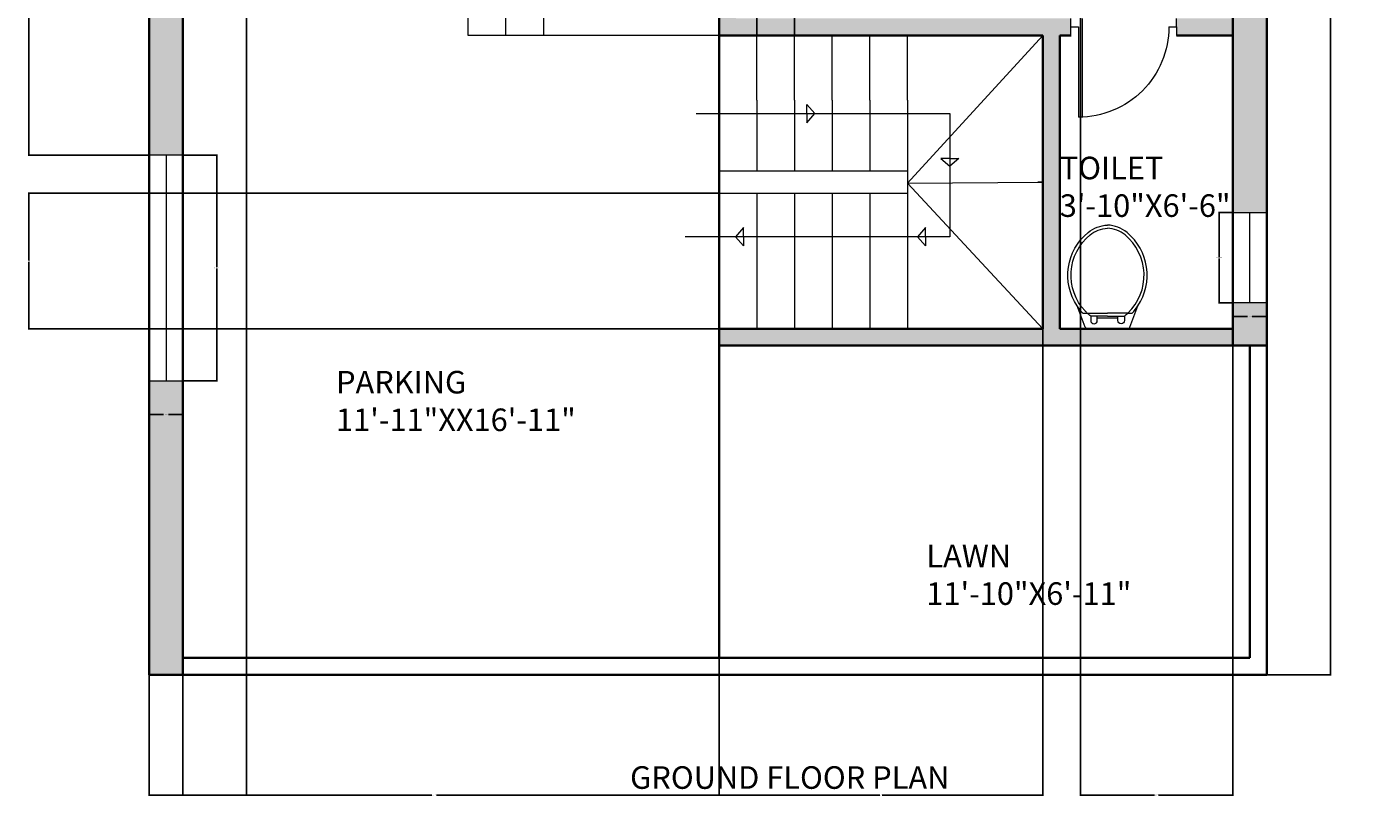
# Model space of a CAD drawing. Units: inches. Extents: x -13 to 349, y -556 to 61.
# Tile 1 of 6: x -13 to 345, y -556 to -351. Entities that reach past the tile are written whole.
import ezdxf

# ---------------------------------------------------------------- set-up
doc = ezdxf.new("R2010")
doc.units = ezdxf.units.IN
doc.header["$MEASUREMENT"] = 0
for name, color, linetype, lineweight in [('A-ANNO-DIMS', 2, 'Continuous', 18), ('A-ANNO-SYMB', 7, 'Continuous', 13), ('A-ANNO-TEXT', 7, 'Continuous', 25), ('A-AREA-IDEN', 7, 'Continuous', 18), ('A-DOOR', 3, 'Continuous', 20), ('A-FLOR-STRS', 7, 'Continuous', 20), ('A-GLAZ', 5, 'Continuous', 18), ('A-WALL', 7, 'Continuous', 35), ('A-WALL-PATT', 8, 'Continuous', 13), ('WC-Detail_dwgmodels.com', 251, 'Continuous', 13), ('WC-Outline_dwgmodels.com', 250, 'Continuous', 18)]:
    doc.layers.add(name, color=color, linetype=linetype, lineweight=lineweight)
doc.styles.get("Standard").update_dxf_attribs({"font": 'arial.ttf'})
doc.dimstyles.get("Standard").update_dxf_attribs({"dimtxt": 0.18, "dimasz": 0.18, "dimexe": 0.18, "dimexo": 0.0625, "dimgap": 0.09, "dimtad": 0, "dimtih": 1, "dimtoh": 1, "dimdec": 0, "dimzin": 0, "dimdsep": 46, "dimlunit": 3, "dimtxsty": 'Standard', "dimcen": 0.09, "dimadec": 0, "dimazin": 0, "dimtfac": 1, "dimtdec": 0, "dimtofl": 0, "dimtmove": 0, "dimatfit": 3, "dimfxl": 1, "dimtolj": 1, "dimtzin": 0, "dimarcsym": 0})

# ---------------------------------------------------------------- blocks, each defined once
blk = doc.blocks.new('*D3')
at = {"layer": 'A-ANNO-DIMS', "color": 0, "lineweight": -2, "transparency": 16777216}
for p, q in [((316.82, 8.29), (333.9, 8.29)), ((333.72, 8.11), (333.72, -254.62)), ((333.72, -523.53), (333.72, -260.8)), ((316.82, -523.71), (333.9, -523.71))]:
    blk.add_line(p, q, dxfattribs=at)
at = {"layer": 'A-ANNO-DIMS', "color": 0, "transparency": 16777216}
for points in [[(333.69, 8.11), (333.75, 8.11), (333.72, 8.29)], [(333.69, -523.53), (333.75, -523.53), (333.72, -523.71)]]:
    blk.add_solid(points, dxfattribs=at)
at = {"layer": 'Defpoints', "color": 0, "transparency": 16777216}
for p in [(316.76, 8.29), (316.76, -523.71), (333.72, -523.71)]:
    blk.add_point(p, dxfattribs=at)
at = {"layer": 'A-ANNO-DIMS', "color": 0, "transparency": 16777216, "insert": (333.72, -257.71), "char_height": 6, "attachment_point": 5}
blk.add_mtext('\\A1;44\'-4"', dxfattribs=at)
blk = doc.blocks.new('DOOR-SWING-24IN')
for p, q in [((4.5, 28), (0, 28)), ((2.25, 28), (2.25, 26)), ((2.25, 26), (26.25, 26)), ((0, 25), (26.25, 25)), ((2.25, 2), (2.25, 0)), ((2.25, 0), (0, 0)), ((2.25, 0), (4.5, 0))]:
    blk.add_line(p, q)
blk.add_arc((2.25, 26), 24, 270, 0)
blk = doc.blocks.new('WIN-60IN-D9')
for p, q in [((0, 60), (0, 0)), ((9, 60), (0, 60)), ((4.5, 60), (4.5, 0)), ((9, 0), (9, 60)), ((0, 0), (9, 0))]:
    blk.add_line(p, q)
blk = doc.blocks.new('WIN-24IN-D9')
for p, q in [((0, 9), (24, 9)), ((0, 0), (0, 9)), ((24, 9), (24, 0)), ((0, 4.5), (24, 4.5)), ((24, 0), (0, 0))]:
    blk.add_line(p, q)
blk = doc.blocks.new('STAIR-DIRECTION-HEAD')
for p, q in [((2.12, 4.81), (0, 2.4)), ((2.12, 2.4), (2.12, 4.81)), ((2.12, 0), (0, 2.4)), ((2.12, 2.4), (2.12, 0))]:
    blk.add_line(p, q)
blk = doc.blocks.new('*D18')
at = {"layer": 'A-ANNO-DIMS', "color": 0, "lineweight": -2, "transparency": 16777216}
for p, q in [((28.82, -385.56), (37.94, -385.56)), ((37.76, -385.74), (37.76, -415.38)), ((37.76, -445.38), (37.76, -415.74)), ((28.82, -445.56), (37.94, -445.56))]:
    blk.add_line(p, q, dxfattribs=at)
at = {"layer": 'A-ANNO-DIMS', "color": 0, "transparency": 16777216}
for points in [[(37.73, -385.74), (37.79, -385.74), (37.76, -385.56)], [(37.73, -445.38), (37.79, -445.38), (37.76, -445.56)]]:
    blk.add_solid(points, dxfattribs=at)
at = {"layer": 'Defpoints', "color": 0, "transparency": 16777216}
for p in [(28.76, -385.56), (37.76, -385.56), (28.76, -445.56)]:
    blk.add_point(p, dxfattribs=at)
at = {"layer": 'A-ANNO-DIMS', "color": 0, "transparency": 16777216, "insert": (37.76, -415.56), "char_height": 0.18, "attachment_point": 5}
blk.add_mtext('\\A1;W1 5\'-0" TYP.', dxfattribs=at)
blk = doc.blocks.new('*D19')
at = {"layer": 'A-ANNO-DIMS', "color": 0, "lineweight": -2, "transparency": 16777216}
for p, q in [((19.76, -445.62), (19.76, -454.74)), ((28.76, -445.62), (28.76, -454.74)), ((19.94, -454.56), (23.62, -454.56)), ((28.58, -454.56), (24.89, -454.56))]:
    blk.add_line(p, q, dxfattribs=at)
at = {"layer": 'A-ANNO-DIMS', "color": 0, "transparency": 16777216}
for points in [[(19.94, -454.53), (19.94, -454.59), (19.76, -454.56)], [(28.58, -454.53), (28.58, -454.59), (28.76, -454.56)]]:
    blk.add_solid(points, dxfattribs=at)
at = {"layer": 'Defpoints', "color": 0, "transparency": 16777216}
for p in [(19.76, -445.56), (28.76, -445.56), (28.76, -454.56)]:
    blk.add_point(p, dxfattribs=at)
at = {"layer": 'A-ANNO-DIMS', "color": 0, "transparency": 16777216, "insert": (24.26, -454.56), "char_height": 0.18, "attachment_point": 5}
blk.add_mtext('\\A1;0\'-9" TYP.', dxfattribs=at)
blk = doc.blocks.new('*D20')
at = {"layer": 'A-ANNO-DIMS', "color": 0, "lineweight": -2, "transparency": 16777216}
for p, q in [((307.69, -400.85), (303.98, -400.85)), ((304.16, -401.03), (304.16, -412.67)), ((304.16, -424.67), (304.16, -413.03)), ((307.69, -424.85), (303.98, -424.85))]:
    blk.add_line(p, q, dxfattribs=at)
at = {"layer": 'A-ANNO-DIMS', "color": 0, "transparency": 16777216}
for points in [[(304.13, -401.03), (304.19, -401.03), (304.16, -400.85)], [(304.13, -424.67), (304.19, -424.67), (304.16, -424.85)]]:
    blk.add_solid(points, dxfattribs=at)
at = {"layer": 'Defpoints', "color": 0, "transparency": 16777216}
for p in [(304.16, -400.85), (307.76, -400.85), (307.76, -424.85)]:
    blk.add_point(p, dxfattribs=at)
at = {"layer": 'A-ANNO-DIMS', "color": 0, "transparency": 16777216, "insert": (304.16, -412.85), "char_height": 0.18, "attachment_point": 5}
blk.add_mtext('\\A1;W2 2\'-0" TYP.', dxfattribs=at)
blk = doc.blocks.new('*D21')
at = {"layer": 'A-ANNO-DIMS', "color": 0, "lineweight": -2, "transparency": 16777216}
for p, q in [((307.76, -424.91), (307.76, -428.63)), ((316.76, -424.91), (316.76, -428.63)), ((307.94, -428.45), (311.62, -428.45)), ((316.58, -428.45), (312.89, -428.45))]:
    blk.add_line(p, q, dxfattribs=at)
at = {"layer": 'A-ANNO-DIMS', "color": 0, "transparency": 16777216}
for points in [[(307.94, -428.42), (307.94, -428.48), (307.76, -428.45)], [(316.58, -428.42), (316.58, -428.48), (316.76, -428.45)]]:
    blk.add_solid(points, dxfattribs=at)
at = {"layer": 'Defpoints', "color": 0, "transparency": 16777216}
for p in [(307.76, -424.85), (316.76, -424.85), (307.76, -428.45)]:
    blk.add_point(p, dxfattribs=at)
at = {"layer": 'A-ANNO-DIMS', "color": 0, "transparency": 16777216, "insert": (312.26, -428.45), "char_height": 0.18, "attachment_point": 5}
blk.add_mtext('\\A1;0\'-9" TYP.', dxfattribs=at)
blk = doc.blocks.new('*D34')
at = {"layer": 'A-ANNO-DIMS', "color": 0, "lineweight": -2, "transparency": 16777216}
for p, q in [((267.26, -200.78), (267.26, -555.89)), ((307.76, -200.78), (307.76, -555.89)), ((267.44, -555.71), (286.97, -555.71)), ((307.58, -555.71), (288.04, -555.71))]:
    blk.add_line(p, q, dxfattribs=at)
at = {"layer": 'A-ANNO-DIMS', "color": 0, "transparency": 16777216}
for points in [[(267.44, -555.68), (267.44, -555.74), (267.26, -555.71)], [(307.58, -555.68), (307.58, -555.74), (307.76, -555.71)]]:
    blk.add_solid(points, dxfattribs=at)
at = {"layer": 'Defpoints', "color": 0, "transparency": 16777216}
for p in [(267.26, -200.71), (307.76, -200.71), (307.76, -555.71)]:
    blk.add_point(p, dxfattribs=at)
at = {"layer": 'A-ANNO-DIMS', "color": 0, "transparency": 16777216, "insert": (287.51, -555.71), "char_height": 0.18, "attachment_point": 5}
blk.add_mtext('\\A1;3\'-4 1/2"', dxfattribs=at)
blk = doc.blocks.new('*D35')
at = {"layer": 'A-ANNO-DIMS', "color": 0, "lineweight": -2, "transparency": 16777216}
for p, q in [((171.26, -431.78), (171.26, -555.89)), ((257.26, -431.78), (257.26, -555.89)), ((171.44, -555.71), (213.93, -555.71)), ((257.08, -555.71), (214.58, -555.71))]:
    blk.add_line(p, q, dxfattribs=at)
at = {"layer": 'A-ANNO-DIMS', "color": 0, "transparency": 16777216}
for points in [[(171.44, -555.68), (171.44, -555.74), (171.26, -555.71)], [(257.08, -555.68), (257.08, -555.74), (257.26, -555.71)]]:
    blk.add_solid(points, dxfattribs=at)
at = {"layer": 'Defpoints', "color": 0, "transparency": 16777216}
for p in [(171.26, -431.71), (257.26, -431.71), (257.26, -555.71)]:
    blk.add_point(p, dxfattribs=at)
at = {"layer": 'A-ANNO-DIMS', "color": 0, "transparency": 16777216, "insert": (214.26, -555.71), "char_height": 0.18, "attachment_point": 5}
blk.add_mtext('\\A1;7\'-2"', dxfattribs=at)
blk = doc.blocks.new('*D36')
at = {"layer": 'A-ANNO-DIMS', "color": 0, "lineweight": -2, "transparency": 16777216}
for p, q in [((171.19, -395.71), (-12.42, -395.71)), ((-12.24, -395.89), (-12.24, -413.53)), ((-12.24, -431.53), (-12.24, -413.9)), ((171.19, -431.71), (-12.42, -431.71))]:
    blk.add_line(p, q, dxfattribs=at)
at = {"layer": 'A-ANNO-DIMS', "color": 0, "transparency": 16777216}
for points in [[(-12.27, -395.89), (-12.21, -395.89), (-12.24, -395.71)], [(-12.27, -431.53), (-12.21, -431.53), (-12.24, -431.71)]]:
    blk.add_solid(points, dxfattribs=at)
at = {"layer": 'Defpoints', "color": 0, "transparency": 16777216}
for p in [(-12.24, -395.71), (171.26, -395.71), (171.26, -431.71)]:
    blk.add_point(p, dxfattribs=at)
at = {"layer": 'A-ANNO-DIMS', "color": 0, "transparency": 16777216, "insert": (-12.24, -413.71), "char_height": 0.18, "attachment_point": 5}
blk.add_mtext('\\A1;3\'-0"', dxfattribs=at)
blk = doc.blocks.new('*D37')
at = {"layer": 'A-ANNO-DIMS', "color": 0, "lineweight": -2, "transparency": 16777216}
for p, q in [((181.26, -353.65), (181.26, 40.47)), ((181.44, 40.29), (185.86, 40.29)), ((191.08, 40.29), (186.65, 40.29)), ((191.26, -353.65), (191.26, 40.47))]:
    blk.add_line(p, q, dxfattribs=at)
at = {"layer": 'A-ANNO-DIMS', "color": 0, "transparency": 16777216}
for points in [[(181.44, 40.32), (181.44, 40.26), (181.26, 40.29)], [(191.08, 40.32), (191.08, 40.26), (191.26, 40.29)]]:
    blk.add_solid(points, dxfattribs=at)
at = {"layer": 'Defpoints', "color": 0, "transparency": 16777216}
for p in [(191.26, 40.29), (181.26, -353.71), (191.26, -353.71)]:
    blk.add_point(p, dxfattribs=at)
at = {"layer": 'A-ANNO-DIMS', "color": 0, "transparency": 16777216, "insert": (186.26, 40.29), "char_height": 0.18, "attachment_point": 5}
blk.add_mtext('\\A1;0\'-10"', dxfattribs=at)
blk = doc.blocks.new('*D38')
at = {"layer": 'A-ANNO-DIMS', "color": 0, "lineweight": -2, "transparency": 16777216}
for p, q in [((28.76, -144.78), (28.76, -555.89)), ((45.63, -144.78), (45.63, -555.89)), ((28.94, -555.71), (36.87, -555.71)), ((45.45, -555.71), (37.51, -555.71))]:
    blk.add_line(p, q, dxfattribs=at)
at = {"layer": 'A-ANNO-DIMS', "color": 0, "transparency": 16777216}
for points in [[(28.94, -555.68), (28.94, -555.74), (28.76, -555.71)], [(45.45, -555.68), (45.45, -555.74), (45.63, -555.71)]]:
    blk.add_solid(points, dxfattribs=at)
at = {"layer": 'Defpoints', "color": 0, "transparency": 16777216}
for p in [(28.76, -144.71), (45.63, -144.71), (45.63, -555.71)]:
    blk.add_point(p, dxfattribs=at)
at = {"layer": 'A-ANNO-DIMS', "color": 0, "transparency": 16777216, "insert": (37.19, -555.71), "char_height": 0.18, "attachment_point": 5}
blk.add_mtext('\\A1;1\'-5"', dxfattribs=at)
blk = doc.blocks.new('*D46')
at = {"layer": 'A-ANNO-DIMS', "color": 0, "lineweight": -2, "transparency": 16777216}
for p, q in [((19.69, -307.06), (-12.42, -307.06)), ((-12.24, -307.24), (-12.24, -346.13)), ((-12.24, -385.38), (-12.24, -346.49)), ((19.69, -385.56), (-12.42, -385.56))]:
    blk.add_line(p, q, dxfattribs=at)
at = {"layer": 'A-ANNO-DIMS', "color": 0, "transparency": 16777216}
for points in [[(-12.27, -307.24), (-12.21, -307.24), (-12.24, -307.06)], [(-12.27, -385.38), (-12.21, -385.38), (-12.24, -385.56)]]:
    blk.add_solid(points, dxfattribs=at)
at = {"layer": 'Defpoints', "color": 0, "transparency": 16777216}
for p in [(19.76, -307.06), (-12.24, -385.56), (19.76, -385.56)]:
    blk.add_point(p, dxfattribs=at)
at = {"layer": 'A-ANNO-DIMS', "color": 0, "transparency": 16777216, "insert": (-12.24, -346.31), "char_height": 0.18, "attachment_point": 5}
blk.add_mtext('\\A1;6\'-6 1/2"', dxfattribs=at)
blk = doc.blocks.new('*D47')
at = {"layer": 'A-ANNO-DIMS', "color": 0, "lineweight": -2, "transparency": 16777216}
for p, q in [((171.26, -519.28), (171.26, -555.89)), ((19.76, -523.78), (19.76, -555.89)), ((19.94, -555.71), (94.91, -555.71)), ((171.08, -555.71), (96.11, -555.71))]:
    blk.add_line(p, q, dxfattribs=at)
at = {"layer": 'A-ANNO-DIMS', "color": 0, "transparency": 16777216}
for points in [[(19.94, -555.68), (19.94, -555.74), (19.76, -555.71)], [(171.08, -555.68), (171.08, -555.74), (171.26, -555.71)]]:
    blk.add_solid(points, dxfattribs=at)
at = {"layer": 'Defpoints', "color": 0, "transparency": 16777216}
for p in [(171.26, -519.21), (19.76, -523.71), (171.26, -555.71)]:
    blk.add_point(p, dxfattribs=at)
at = {"layer": 'A-ANNO-DIMS', "color": 0, "transparency": 16777216, "insert": (95.51, -555.71), "char_height": 0.18, "attachment_point": 5}
blk.add_mtext('\\A1;12\'-7 1/2"', dxfattribs=at)

msp = doc.modelspace()

# ---------------------------------------------------------------- hatches: boundary and pattern name
at = {"layer": 'A-WALL-PATT'}
h = msp.add_hatch(color=256, dxfattribs=at)
h.dxf.hatch_style = 1
h.paths.add_polyline_path([(316.76, 8.29), (171.26, 8.29), (171.26, -0.71), (307.76, -0.71), (307.76, -52.19), (316.76, -52.19)])
h.paths.add_polyline_path([(175.76, -0.71), (171.26, -0.71), (171.26, -82.21), (165.24, -82.21), (165.24, -86.71), (171.26, -86.71), (171.26, -101.71), (173.51, -101.71), (175.76, -101.71)])
h.paths.add_polyline_path([(171.26, -25.21), (165.17, -25.21), (165.17, -34.21), (171.26, -34.21)])
h.paths.add_polyline_path([(141.17, -25.21), (127.76, -25.21), (127.76, -34.21), (141.17, -34.21)])
h.paths.add_polyline_path([(28.76, -25.21), (24.26, -25.21), (19.76, -25.21), (19.76, -78.88), (28.76, -78.88)])
h.paths.add_polyline_path([(99.76, -29.71), (99.76, -25.21), (28.76, -25.21), (28.76, -34.21), (99.76, -34.21)])
h.paths.add_polyline_path([(135.26, -86.71), (143.68, -86.71), (143.68, -82.21), (135.26, -82.21), (135.26, -34.21), (130.76, -34.21), (130.76, -101.71), (133.01, -101.71), (135.26, -101.71)])
h.paths.add_polyline_path([(135.26, -141.71), (130.76, -141.71), (130.76, -144.71), (28.76, -144.71), (28.76, -149.21), (135.26, -149.21)])
h.paths.add_polyline_path([(28.76, -138.88), (19.76, -138.88), (19.76, -156.62), (28.76, -156.62)])
h.paths.add_polyline_path([(28.76, -192.62), (19.76, -192.62), (19.76, -271.06), (28.76, -271.06)])
h.paths.add_polyline_path([(28.76, -307.06), (19.76, -307.06), (19.76, -385.56), (28.76, -385.56)])
h.paths.add_polyline_path([(28.76, -445.56), (19.76, -445.56), (19.76, -523.71), (28.76, -523.71)])
h.paths.add_polyline_path([(307.76, -431.71), (261.76, -431.71), (261.76, -353.71), (264.76, -353.71), (264.76, -349.21), (175.76, -349.21), (175.76, -248.21), (173.51, -248.21), (171.26, -248.21), (171.26, -317.21), (168.26, -317.21), (168.26, -321.71), (171.26, -321.71), (171.26, -353.71), (257.26, -353.71), (257.26, -431.71), (171.26, -431.71), (171.26, -436.21), (307.76, -436.21)])
h.paths.add_polyline_path([(316.76, -424.85), (307.76, -424.85), (307.76, -436.21), (316.76, -436.21)])
h.paths.add_polyline_path([(316.76, -305.84), (307.76, -305.84), (307.76, -400.85), (316.76, -400.85)])
h.paths.add_polyline_path([(307.76, -349.21), (292.76, -349.21), (292.76, -351.46), (292.76, -353.71), (307.76, -353.71)], flags=17)
h.paths.add_polyline_path([(271.19, -200.71), (267.26, -200.71), (267.26, -186.96), (262.76, -186.96), (262.76, -200.71), (175.76, -200.71), (175.76, -180.21), (173.51, -180.21), (171.26, -180.21), (171.26, -208.21), (175.76, -208.21), (175.76, -205.21), (271.19, -205.21)])
h.paths.add_polyline_path([(316.76, -112.19), (307.76, -112.19), (307.76, -245.84), (316.76, -245.84)])
h.paths.add_polyline_path([(271.33, -144.71), (175.76, -144.71), (175.76, -141.71), (171.26, -141.71), (171.26, -152.21), (175.76, -152.21), (175.76, -149.21), (262.76, -149.21), (262.76, -162.96), (267.26, -162.96), (267.26, -149.21), (271.33, -149.21)])
h.paths.add_polyline_path([(307.76, -200.71), (307.19, -200.71), (307.19, -205.21), (307.76, -205.21)])
h.paths.add_polyline_path([(307.76, -144.71), (307.33, -144.71), (307.33, -149.21), (307.76, -149.21)])

# ---------------------------------------------------------------- linework, layer by layer
at = {"layer": 'A-ANNO-SYMB'}
for p, q in [((165.11, -374.53), (232.53, -374.53)), ((232.53, -374.53), (232.53, -407.24)), ((232.53, -407.24), (162.25, -407.24))]:
    msp.add_line(p, q, dxfattribs=at)
at = {"layer": 'A-FLOR-STRS'}
for p, q in [((104.53, -353.71), (104.53, -321.71)), ((114.53, -353.71), (114.53, -321.71)), ((124.53, -321.71), (124.53, -353.71)), ((114.53, -353.71), (104.53, -353.71)), ((124.53, -353.71), (114.53, -353.71)), ((171.26, -353.71), (124.53, -353.71)), ((181.26, -370.98), (181.26, -353.71)), ((191.26, -370.98), (191.26, -353.71)), ((201.26, -370.98), (201.26, -353.71)), ((211.26, -370.98), (211.26, -353.71)), ((221.26, -370.98), (221.26, -353.71)), ((221.26, -393.01), (257.26, -353.71)), ((181.26, -370.98), (181.26, -389.71)), ((191.26, -370.98), (191.26, -389.71)), ((201.26, -370.98), (201.26, -389.71)), ((211.26, -370.98), (211.26, -389.71)), ((221.26, -370.98), (221.26, -431.71)), ((171.26, -389.71), (221.26, -389.71)), ((221.26, -393.01), (257.26, -392.71)), ((221.26, -393.01), (257.26, -431.71)), ((257.26, -392.71), (255.95, -392.71)), ((171.26, -395.71), (221.26, -395.71)), ((181.26, -395.71), (181.26, -431.71)), ((191.26, -395.71), (191.26, -431.71)), ((201.26, -395.71), (201.26, -431.71)), ((211.26, -395.71), (211.26, -431.71))]:
    msp.add_line(p, q, dxfattribs=at)
at = {"layer": 'A-WALL'}
for p, q in [((19.76, 8.29), (19.76, -523.71)), ((316.76, 8.29), (316.76, -523.71)), ((307.76, -0.71), (307.76, -436.21)), ((28.76, -25.21), (28.76, -523.71)), ((171.26, -321.71), (171.26, -519.21)), ((171.26, -353.71), (257.26, -353.71)), ((257.26, -353.71), (257.26, -431.71)), ((261.76, -353.71), (264.76, -353.71)), ((261.76, -353.71), (261.76, -431.71)), ((292.76, -353.71), (307.76, -353.71)), ((171.26, -431.71), (257.26, -431.71)), ((261.76, -431.71), (307.76, -431.71)), ((171.26, -436.21), (307.76, -436.21)), ((307.76, -436.21), (316.76, -436.21)), ((312.26, -436.21), (312.26, -519.21)), ((28.76, -519.21), (307.76, -519.21)), ((312.26, -519.21), (307.76, -519.21)), ((19.76, -523.71), (316.76, -523.71))]:
    msp.add_line(p, q, dxfattribs=at)
at = {"layer": 'WC-Detail_dwgmodels.com'}
for p, q in [((267.89, -427.54), (269.04, -427.54)), ((279.89, -427.54), (281.04, -427.54))]:
    msp.add_line(p, q, dxfattribs=at)
for points in [[(267.89, -427.54, -0.040937), (266.39, -425.65, -0.163732)], [(281.04, -427.54, 0.040937), (282.53, -425.65, 0.163732)], [(269.99, -428.37, -0.022712), (269.04, -427.54, -0.162618)], [(274.46, -428.37), (269.99, -428.37, -0.022712)], [(269.99, -428.37), (269.99, -429.53, 1), (271.75, -429.53), (271.75, -428.93)], [(274.46, -428.37), (278.94, -428.37, 0.476108)], [(278.94, -428.37), (278.94, -429.53, -1), (277.18, -429.53), (277.18, -428.93)], [(278.94, -428.37, 0.022712), (279.89, -427.54, 0.162618)]]:
    msp.add_lwpolyline(points, format="xyb", dxfattribs=at)
for points in [[(271.75, -428.93), (271.75, -428.37)], [(277.18, -428.93), (271.75, -428.93)], [(277.18, -428.93), (277.18, -428.37)]]:
    msp.add_lwpolyline(points, dxfattribs=at)
at = {"layer": 'WC-Outline_dwgmodels.com'}
for p in [(269.04, -427.54), (279.89, -427.54)]:
    msp.add_line(p, (274.46, -427.54), dxfattribs=at)
for points in [[(266.39, -425.65, -0.383919), (269.28, -406.14, -0.163732), (274.46, -404.15, -0.359733)], [(282.53, -425.65, 0.383919), (279.64, -406.14, 0.163732), (274.46, -404.15, 0.359733)], [(268.49, -426.98, -0.431639), (269.81, -406.77, -0.162618), (274.46, -404.98, -0.470877)], [(279.89, -427.54, 0.448546), (279.12, -406.77, 0.162618), (274.46, -404.98, 0.470877)], [(274.46, -431.71), (269.2, -431.71, -0.31031), (268.56, -431.27), (266.39, -425.65, -0.209071)], [(274.46, -431.71), (279.73, -431.71, 0.31031), (280.37, -431.27), (282.53, -425.65, 0.209071)], [(269.04, -427.54, -0.014165), (268.49, -426.98, -0.162618)]]:
    msp.add_lwpolyline(points, format="xyb", dxfattribs=at)

# ---------------------------------------------------------------- block references
at = {"layer": 'A-ANNO-SYMB'}
for p, rotation in [((196.71, -372.13), 180), ((234.93, -388.53), 90.04341119574104)]:
    msp.add_blockref('STAIR-DIRECTION-HEAD', p, dxfattribs=dict(at, rotation=rotation))
for p in [(175.56, -409.64), (223.95, -409.64)]:
    msp.add_blockref('STAIR-DIRECTION-HEAD', p, dxfattribs=at)
at = {"layer": 'A-DOOR', "extrusion": (0, 0, -1), "zscale": -1, "rotation": 269.9999999999996}
msp.add_blockref('DOOR-SWING-24IN', (-292.75, -349.22), dxfattribs=at)
at = {"layer": 'A-GLAZ'}
msp.add_blockref('WIN-60IN-D9', (19.76, -445.56), dxfattribs=at)
at = {"layer": 'A-GLAZ', "rotation": 90.00000000000003}
msp.add_blockref('WIN-24IN-D9', (316.75, -424.85), dxfattribs=at)

# ---------------------------------------------------------------- texts
at = {"layer": 'A-ANNO-TEXT', "insert": (147.58, -548.05), "char_height": 6, "attachment_point": 1}
msp.add_mtext('GROUND FLOOR PLAN', dxfattribs=at)
at = {"layer": 'A-AREA-IDEN', "char_height": 6, "attachment_point": 1}
for s, insert in [('TOILET\\P3\'-10"X6\'-6"', (261.76, -385.98)), ('LAWN\\P11\'-10"X6\'-11"', (226.31, -489.14))]:
    msp.add_mtext(s, dxfattribs=dict(at, insert=insert))
at = {"layer": 'A-AREA-IDEN', "insert": (69.43, -442.93), "char_height": 6, "attachment_point": 1}
msp.add_mtext_dynamic_manual_height_columns('PARKING\\P11\'-11"XX16\'-11"', width=2.3415, gutter_width=1, heights=[0], dxfattribs=at)

# ---------------------------------------------------------------- dimensions: what is measured, and where the dimension line sits
at = {"layer": 'A-ANNO-DIMS'}
for base, p1, p2, picture, middle in [((191.26, 40.29), (181.26, -353.71), (191.26, -353.71), '*D37', (186.26, 40.29)), ((45.63, -555.71), (28.76, -144.71), (45.63, -144.71), '*D38', (37.19, -555.71)), ((307.76, -555.71), (267.26, -200.71), (307.76, -200.71), '*D34', (287.51, -555.71)), ((257.26, -555.71), (171.26, -431.71), (257.26, -431.71), '*D35', (214.26, -555.71)), ((171.26, -555.71), (19.76, -523.71), (171.26, -519.21), '*D47', (95.51, -555.71))]:
    dim = msp.add_linear_dim(base=base, p1=p1, p2=p2, dimstyle='Standard', override={"dimdec": 1, "dimlfac": 1, "dimrnd": 0, "dimzin": 1, "dimdsep": 46, "dimlunit": 4, "dimfrac": 2}, dxfattribs=at)
    dim.commit()
    dim.dimension.update_dxf_attribs({"geometry": picture, "text_midpoint": middle})
for base, p1, p2, override, picture, middle in [((333.72, -523.71), (316.76, 8.29), (316.76, -523.71), {"dimtxt": 6, "dimclrd": 0, "dimclre": 0, "dimclrt": 0}, '*D3', (333.72, -257.71)), ((-12.24, -385.56), (19.76, -307.06), (19.76, -385.56), {"dimdec": 1, "dimlfac": 1, "dimrnd": 0, "dimzin": 1, "dimdsep": 46, "dimlunit": 4, "dimfrac": 2}, '*D46', (-12.24, -346.31)), ((-12.24, -395.71), (171.26, -431.71), (171.26, -395.71), {"dimdec": 1, "dimlfac": 1, "dimrnd": 0, "dimzin": 1, "dimdsep": 46, "dimlunit": 4, "dimfrac": 2}, '*D36', (-12.24, -413.71))]:
    dim = msp.add_linear_dim(base=base, p1=p1, p2=p2, angle=90, dimstyle='Standard', override=override, dxfattribs=at)
    dim.commit()
    dim.dimension.update_dxf_attribs({"geometry": picture, "text_midpoint": middle})
for base, p1, p2, angle, text, picture, middle in [((37.76, -385.56), (28.76, -445.56), (28.76, -385.56), 90, 'W1 <> TYP.', '*D18', (37.76, -415.56)), ((304.16, -400.85), (307.76, -424.85), (307.76, -400.85), 90, 'W2 <> TYP.', '*D20', (304.16, -412.85)), ((307.76, -428.45), (316.76, -424.85), (307.76, -424.85), 180, '<> TYP.', '*D21', (312.26, -428.45))]:
    dim = msp.add_linear_dim(base=base, p1=p1, p2=p2, angle=angle, text=text, dimstyle='Standard', override={"dimdec": 1, "dimlfac": 1, "dimrnd": 0, "dimzin": 1, "dimdsep": 46, "dimlunit": 4, "dimfrac": 2}, dxfattribs=at)
    dim.commit()
    dim.dimension.update_dxf_attribs({"geometry": picture, "text_midpoint": middle})
dim = msp.add_linear_dim(base=(28.76, -454.56), p1=(19.76, -445.56), p2=(28.76, -445.56), text='<> TYP.', dimstyle='Standard', override={"dimdec": 1, "dimlfac": 1, "dimrnd": 0, "dimzin": 1, "dimdsep": 46, "dimlunit": 4, "dimfrac": 2}, dxfattribs=at)
dim.commit()
dim.dimension.update_dxf_attribs({"geometry": '*D19', "text_midpoint": (24.26, -454.56)})

doc.saveas('drawing.dxf')
